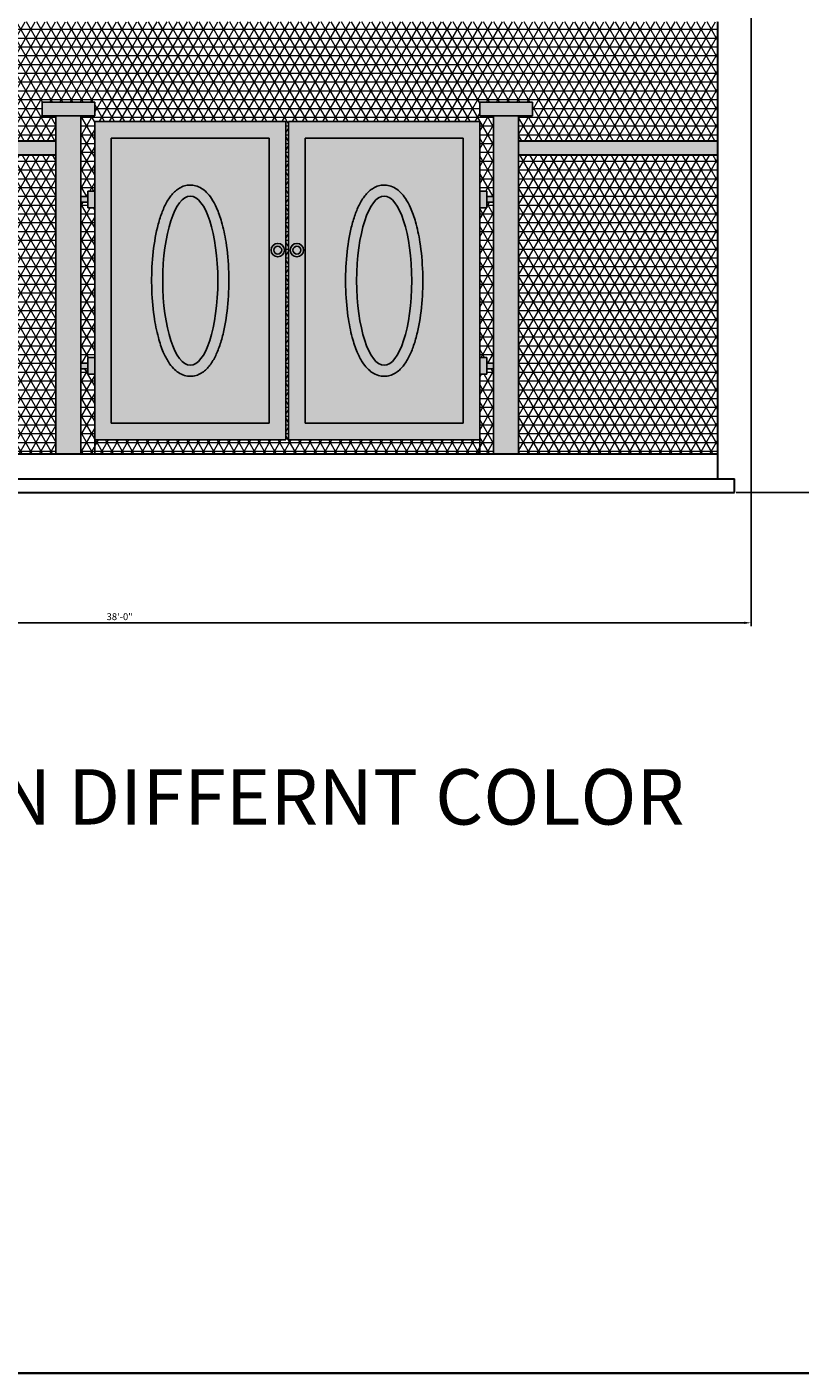
# Model space of a CAD drawing. Units: inches. Extents: x 2391 to 16591, y 7259 to 10239.
# Tile 4 of 27: x 3208 to 3487, y 7259 to 7745. Entities that reach past the tile are written whole.
import ezdxf

# ---------------------------------------------------------------- set-up
doc = ezdxf.new("R2010")
doc.units = ezdxf.units.IN
for name, color, linetype, lineweight in [('A-ANNO-DIMS', 4, 'Continuous', 18), ('A-ANNO-TITL', 3, 'Continuous', 30), ('A-ANNO-TTLB', 7, 'Continuous', 35), ('A-ELEV', 7, 'Continuous', 30), ('A-ELEV-GATE', 7, 'Continuous', 25), ('A-ELEV-GATE-PATT', 252, 'Continuous', 13), ('A-ELEV-PATT', 8, 'Continuous', 13), ('A-ELEV-SURF-PATT', 253, 'Continuous', 13)]:
    doc.layers.add(name, color=color, linetype=linetype, lineweight=lineweight)
doc.styles.get("Standard").update_dxf_attribs({"font": 'arial.ttf'})
doc.dimstyles.new('ISO-25', dxfattribs={"dimtxt": 2.5, "dimasz": 2.5, "dimexe": 1.25, "dimexo": 0.625, "dimtad": 1, "dimdec": 0, "dimlunit": 3, "dimtxsty": 'Standard', "dimcen": 2.5, "dimadec": 0, "dimazin": 0, "dimtfac": 1, "dimtdec": 0, "dimtmove": 0, "dimatfit": 3, "dimfxl": 1, "dimarcsym": 0})

# ---------------------------------------------------------------- blocks, each defined once
blk = doc.blocks.new('GATE-HINGE-ELEV')
for p, q in [((5, 6), (2.5, 6)), ((2.5, 6), (2.5, 0)), ((2.5, 4), (0, 4)), ((2.5, 2), (0, 2)), ((5, 0), (2.5, 0))]:
    blk.add_line(p, q)
blk = doc.blocks.new('*D83')
at = {"layer": 'A-ANNO-DIMS', "color": 0, "lineweight": -2, "transparency": 16777216}
for p, q in [((3013.78, 7751.89), (3013.78, 7528.22)), ((3469.78, 7751.89), (3469.78, 7528.22)), ((3016.28, 7529.47), (3467.28, 7529.47))]:
    blk.add_line(p, q, dxfattribs=at)
at = {"layer": 'A-ANNO-DIMS', "color": 0, "transparency": 16777216}
for points in [[(3016.28, 7529.89), (3016.28, 7529.05), (3013.78, 7529.47)], [(3467.28, 7529.89), (3467.28, 7529.05), (3469.78, 7529.47)]]:
    blk.add_solid(points, dxfattribs=at)
at = {"layer": 'Defpoints', "color": 0, "transparency": 16777216}
for p in [(3013.78, 7752.52), (3469.78, 7752.52), (3469.78, 7529.47)]:
    blk.add_point(p, dxfattribs=at)
at = {"layer": 'A-ANNO-DIMS', "color": 0, "transparency": 16777216, "insert": (3241.78, 7531.37), "char_height": 2.5, "attachment_point": 5}
blk.add_mtext('38\'-0"', dxfattribs=at)
blk = doc.blocks.new('*D84')
at = {"layer": 'A-ANNO-DIMS', "color": 0, "lineweight": -2, "transparency": 16777216}
for p, q in [((3437.4, 8339.52), (3518.08, 8339.52)), ((3516.83, 7579.02), (3516.83, 8337.02)), ((3464.4, 7576.52), (3518.08, 7576.52))]:
    blk.add_line(p, q, dxfattribs=at)
at = {"layer": 'A-ANNO-DIMS', "color": 0, "transparency": 16777216}
for points in [[(3516.41, 8337.02), (3517.24, 8337.02), (3516.83, 8339.52)], [(3516.41, 7579.02), (3517.24, 7579.02), (3516.83, 7576.52)]]:
    blk.add_solid(points, dxfattribs=at)
at = {"layer": 'Defpoints', "color": 0, "transparency": 16777216}
for p in [(3436.78, 8339.52), (3516.83, 8339.52), (3463.78, 7576.52)]:
    blk.add_point(p, dxfattribs=at)
at = {"layer": 'A-ANNO-DIMS', "color": 0, "transparency": 16777216, "insert": (3514.93, 7958.02), "char_height": 2.5, "attachment_point": 5, "rotation": 90}
blk.add_mtext('63\'-7"', dxfattribs=at)

msp = doc.modelspace()

# ---------------------------------------------------------------- hatches: boundary and pattern name
at = {"layer": 'A-ELEV-GATE-PATT'}
h = msp.add_hatch(color=256, dxfattribs=at)
h.dxf.hatch_style = 1
h.paths.add_polyline_path([(3218.78, 7590.52), (3227.78, 7590.52), (3227.78, 7712.52), (3218.78, 7712.52)])
h.paths.add_polyline_path([(3385.78, 7712.52), (3376.78, 7712.52), (3376.78, 7590.52), (3385.78, 7590.52)])
h = msp.add_hatch(color=256, dxfattribs=at)
h.dxf.hatch_style = 1
h.paths.add_polyline_path([(3232.78, 7595.52), (3301.78, 7595.52), (3301.78, 7710.52), (3232.78, 7710.52)])
h.paths.add_polyline_path([(3238.78, 7704.52), (3295.78, 7704.52), (3295.78, 7601.52), (3238.78, 7601.52)], flags=16)
edge = h.paths.add_edge_path(flags=0)
edge.add_spline(control_points=[(3267.28, 7618.48), (3267.98, 7618.48), (3268.69, 7618.59), (3270.01, 7618.97), (3270.63, 7619.25), (3271.76, 7619.93), (3272.28, 7620.32), (3273.23, 7621.18), (3273.67, 7621.64), (3274.89, 7623.14), (3275.59, 7624.27), (3276.85, 7626.76), (3277.41, 7628.13), (3278.43, 7631.09), (3278.88, 7632.69), (3280.01, 7637.55), (3280.54, 7641.06), (3281.19, 7648.39), (3281.29, 7652.22), (3281.06, 7659.76), (3280.73, 7663.47), (3279.77, 7669.53), (3279.25, 7671.99), (3278.08, 7676.08), (3277.48, 7677.78), (3276.25, 7680.54), (3275.65, 7681.66), (3274.42, 7683.5), (3273.83, 7684.25), (3272.61, 7685.46), (3272.01, 7685.95), (3270.68, 7686.77), (3269.94, 7687.11), (3268.5, 7687.48), (3267.83, 7687.57), (3266.48, 7687.55), (3265.81, 7687.44), (3264.54, 7687.06), (3263.95, 7686.8), (3262.86, 7686.16), (3262.36, 7685.79), (3261.44, 7684.98), (3261.02, 7684.54), (3259.81, 7683.1), (3259.11, 7682.01), (3257.84, 7679.59), (3257.28, 7678.26), (3256.26, 7675.38), (3255.81, 7673.83), (3254.67, 7669.1), (3254.11, 7665.68), (3253.42, 7658.51), (3253.28, 7654.75), (3253.43, 7647.32), (3253.72, 7643.64), (3254.6, 7637.46), (3255.12, 7634.88), (3256.27, 7630.6), (3256.87, 7628.82), (3258.1, 7625.93), (3258.7, 7624.75), (3259.92, 7622.82), (3260.52, 7622.04), (3261.74, 7620.77), (3262.33, 7620.25), (3263.67, 7619.38), (3264.41, 7619.01), (3265.88, 7618.59), (3266.58, 7618.48), (3267.28, 7618.48)], knot_values=[0, 0, 0, 0, 0.095196, 0.095196, 0.190392, 0.190392, 0.285588, 0.285588, 0.380784, 0.380784, 0.570897, 0.570897, 0.76101, 0.76101, 0.951123, 0.951123, 1.307609, 1.307609, 1.664096, 1.664096, 2.020583, 2.020583, 2.290036, 2.290036, 2.5108, 2.5108, 2.687191, 2.687191, 2.829292, 2.829292, 2.942747, 2.942747, 3.056202, 3.056202, 3.147245, 3.147245, 3.238288, 3.238288, 3.329331, 3.329331, 3.420374, 3.420374, 3.511418, 3.511418, 3.698581, 3.698581, 3.885745, 3.885745, 4.072908, 4.072908, 4.42383, 4.42383, 4.774752, 4.774752, 5.125674, 5.125674, 5.403289, 5.403289, 5.629501, 5.629501, 5.810378, 5.810378, 5.956164, 5.956164, 6.072402, 6.072402, 6.18864, 6.18864, 6.283185, 6.283185, 6.283185, 6.283185], degree=3, periodic=0)
edge = h.paths.add_edge_path(flags=0)
edge.add_ellipse((3267.28, 7653.02), major_axis=(0, -30.54), ratio=0.325581, start_angle=0, end_angle=360)
h.paths.add_polyline_path([(3300.28, 7664.05, -1), (3297.44, 7664.05, -1)], flags=16)
h.paths.add_polyline_path([(3302.78, 7595.52), (3371.78, 7595.52), (3371.78, 7710.52), (3302.78, 7710.52)])
h.paths.add_polyline_path([(3308.78, 7704.52), (3365.78, 7704.52), (3365.78, 7601.52), (3308.78, 7601.52)], flags=16)
edge = h.paths.add_edge_path(flags=0)
edge.add_spline(control_points=[(3337.28, 7618.48), (3337.98, 7618.48), (3338.69, 7618.59), (3340.01, 7618.97), (3340.63, 7619.25), (3341.76, 7619.93), (3342.28, 7620.32), (3343.23, 7621.18), (3343.67, 7621.64), (3344.89, 7623.14), (3345.59, 7624.27), (3346.85, 7626.76), (3347.41, 7628.13), (3348.43, 7631.09), (3348.88, 7632.69), (3350.01, 7637.55), (3350.54, 7641.06), (3351.19, 7648.39), (3351.29, 7652.22), (3351.06, 7659.76), (3350.73, 7663.47), (3349.77, 7669.53), (3349.25, 7671.99), (3348.08, 7676.08), (3347.48, 7677.78), (3346.25, 7680.54), (3345.65, 7681.66), (3344.42, 7683.5), (3343.83, 7684.25), (3342.61, 7685.46), (3342.01, 7685.95), (3340.68, 7686.77), (3339.94, 7687.11), (3338.5, 7687.48), (3337.83, 7687.57), (3336.48, 7687.55), (3335.81, 7687.44), (3334.54, 7687.06), (3333.95, 7686.8), (3332.86, 7686.16), (3332.36, 7685.79), (3331.44, 7684.98), (3331.02, 7684.54), (3329.81, 7683.1), (3329.11, 7682.01), (3327.84, 7679.59), (3327.28, 7678.26), (3326.26, 7675.38), (3325.81, 7673.83), (3324.67, 7669.1), (3324.11, 7665.68), (3323.42, 7658.51), (3323.28, 7654.75), (3323.43, 7647.32), (3323.72, 7643.64), (3324.6, 7637.46), (3325.12, 7634.88), (3326.27, 7630.6), (3326.87, 7628.82), (3328.1, 7625.93), (3328.7, 7624.75), (3329.92, 7622.82), (3330.52, 7622.04), (3331.74, 7620.77), (3332.33, 7620.25), (3333.67, 7619.38), (3334.41, 7619.01), (3335.88, 7618.59), (3336.58, 7618.48), (3337.28, 7618.48)], knot_values=[0, 0, 0, 0, 0.095196, 0.095196, 0.190392, 0.190392, 0.285588, 0.285588, 0.380784, 0.380784, 0.570897, 0.570897, 0.76101, 0.76101, 0.951123, 0.951123, 1.307609, 1.307609, 1.664096, 1.664096, 2.020583, 2.020583, 2.290036, 2.290036, 2.5108, 2.5108, 2.687191, 2.687191, 2.829292, 2.829292, 2.942747, 2.942747, 3.056202, 3.056202, 3.147245, 3.147245, 3.238288, 3.238288, 3.329331, 3.329331, 3.420374, 3.420374, 3.511418, 3.511418, 3.698581, 3.698581, 3.885745, 3.885745, 4.072908, 4.072908, 4.42383, 4.42383, 4.774752, 4.774752, 5.125674, 5.125674, 5.403289, 5.403289, 5.629501, 5.629501, 5.810378, 5.810378, 5.956164, 5.956164, 6.072402, 6.072402, 6.18864, 6.18864, 6.283185, 6.283185, 6.283185, 6.283185], degree=3, periodic=0)
edge = h.paths.add_edge_path(flags=0)
edge.add_ellipse((3337.28, 7653.02), major_axis=(0, -30.54), ratio=0.325581, start_angle=0, end_angle=360)
h.paths.add_polyline_path([(3308.19, 7664.05, -1), (3303.36, 7664.05, -1)], flags=16)
h.paths.add_polyline_path([(3307.19, 7664.05, -1), (3304.36, 7664.05, -1)], flags=0)
h = msp.add_hatch(color=256, dxfattribs=at)
h.dxf.hatch_style = 1
h.paths.add_polyline_path([(3238.78, 7704.52), (3238.78, 7601.52), (3295.78, 7601.52), (3295.78, 7704.52)])
edge = h.paths.add_edge_path(flags=16)
edge.add_spline(control_points=[(3267.28, 7618.48), (3267.98, 7618.48), (3268.69, 7618.59), (3270.01, 7618.97), (3270.63, 7619.25), (3271.76, 7619.93), (3272.28, 7620.32), (3273.23, 7621.18), (3273.67, 7621.64), (3274.89, 7623.14), (3275.59, 7624.27), (3276.85, 7626.76), (3277.41, 7628.13), (3278.43, 7631.09), (3278.88, 7632.69), (3280.01, 7637.55), (3280.54, 7641.06), (3281.19, 7648.39), (3281.29, 7652.22), (3281.06, 7659.76), (3280.73, 7663.47), (3279.77, 7669.53), (3279.25, 7671.99), (3278.08, 7676.08), (3277.48, 7677.78), (3276.25, 7680.54), (3275.65, 7681.66), (3274.42, 7683.5), (3273.83, 7684.25), (3272.61, 7685.46), (3272.01, 7685.95), (3270.68, 7686.77), (3269.94, 7687.11), (3268.5, 7687.48), (3267.83, 7687.57), (3266.48, 7687.55), (3265.81, 7687.44), (3264.54, 7687.06), (3263.95, 7686.8), (3262.86, 7686.16), (3262.36, 7685.79), (3261.44, 7684.98), (3261.02, 7684.54), (3259.81, 7683.1), (3259.11, 7682.01), (3257.84, 7679.59), (3257.28, 7678.26), (3256.26, 7675.38), (3255.81, 7673.83), (3254.67, 7669.1), (3254.11, 7665.68), (3253.42, 7658.51), (3253.28, 7654.75), (3253.43, 7647.32), (3253.72, 7643.64), (3254.6, 7637.46), (3255.12, 7634.88), (3256.27, 7630.6), (3256.87, 7628.82), (3258.1, 7625.93), (3258.7, 7624.75), (3259.92, 7622.82), (3260.52, 7622.04), (3261.74, 7620.77), (3262.33, 7620.25), (3263.67, 7619.38), (3264.41, 7619.01), (3265.88, 7618.59), (3266.58, 7618.48), (3267.28, 7618.48)], knot_values=[0, 0, 0, 0, 0.095196, 0.095196, 0.190392, 0.190392, 0.285588, 0.285588, 0.380784, 0.380784, 0.570897, 0.570897, 0.76101, 0.76101, 0.951123, 0.951123, 1.307609, 1.307609, 1.664096, 1.664096, 2.020583, 2.020583, 2.290036, 2.290036, 2.5108, 2.5108, 2.687191, 2.687191, 2.829292, 2.829292, 2.942747, 2.942747, 3.056202, 3.056202, 3.147245, 3.147245, 3.238288, 3.238288, 3.329331, 3.329331, 3.420374, 3.420374, 3.511418, 3.511418, 3.698581, 3.698581, 3.885745, 3.885745, 4.072908, 4.072908, 4.42383, 4.42383, 4.774752, 4.774752, 5.125674, 5.125674, 5.403289, 5.403289, 5.629501, 5.629501, 5.810378, 5.810378, 5.956164, 5.956164, 6.072402, 6.072402, 6.18864, 6.18864, 6.283185, 6.283185, 6.283185, 6.283185], degree=3, periodic=0)
edge = h.paths.add_edge_path(flags=0)
edge.add_ellipse((3267.28, 7653.02), major_axis=(0, -30.54), ratio=0.325581, start_angle=0, end_angle=360)
h.paths.add_polyline_path([(3308.78, 7704.52), (3308.78, 7601.52), (3365.78, 7601.52), (3365.78, 7704.52)])
edge = h.paths.add_edge_path(flags=16)
edge.add_spline(control_points=[(3337.28, 7618.48), (3337.98, 7618.48), (3338.69, 7618.59), (3340.01, 7618.97), (3340.63, 7619.25), (3341.76, 7619.93), (3342.28, 7620.32), (3343.23, 7621.18), (3343.67, 7621.64), (3344.89, 7623.14), (3345.59, 7624.27), (3346.85, 7626.76), (3347.41, 7628.13), (3348.43, 7631.09), (3348.88, 7632.69), (3350.01, 7637.55), (3350.54, 7641.06), (3351.19, 7648.39), (3351.29, 7652.22), (3351.06, 7659.76), (3350.73, 7663.47), (3349.77, 7669.53), (3349.25, 7671.99), (3348.08, 7676.08), (3347.48, 7677.78), (3346.25, 7680.54), (3345.65, 7681.66), (3344.42, 7683.5), (3343.83, 7684.25), (3342.61, 7685.46), (3342.01, 7685.95), (3340.68, 7686.77), (3339.94, 7687.11), (3338.5, 7687.48), (3337.83, 7687.57), (3336.48, 7687.55), (3335.81, 7687.44), (3334.54, 7687.06), (3333.95, 7686.8), (3332.86, 7686.16), (3332.36, 7685.79), (3331.44, 7684.98), (3331.02, 7684.54), (3329.81, 7683.1), (3329.11, 7682.01), (3327.84, 7679.59), (3327.28, 7678.26), (3326.26, 7675.38), (3325.81, 7673.83), (3324.67, 7669.1), (3324.11, 7665.68), (3323.42, 7658.51), (3323.28, 7654.75), (3323.43, 7647.32), (3323.72, 7643.64), (3324.6, 7637.46), (3325.12, 7634.88), (3326.27, 7630.6), (3326.87, 7628.82), (3328.1, 7625.93), (3328.7, 7624.75), (3329.92, 7622.82), (3330.52, 7622.04), (3331.74, 7620.77), (3332.33, 7620.25), (3333.67, 7619.38), (3334.41, 7619.01), (3335.88, 7618.59), (3336.58, 7618.48), (3337.28, 7618.48)], knot_values=[0, 0, 0, 0, 0.095196, 0.095196, 0.190392, 0.190392, 0.285588, 0.285588, 0.380784, 0.380784, 0.570897, 0.570897, 0.76101, 0.76101, 0.951123, 0.951123, 1.307609, 1.307609, 1.664096, 1.664096, 2.020583, 2.020583, 2.290036, 2.290036, 2.5108, 2.5108, 2.687191, 2.687191, 2.829292, 2.829292, 2.942747, 2.942747, 3.056202, 3.056202, 3.147245, 3.147245, 3.238288, 3.238288, 3.329331, 3.329331, 3.420374, 3.420374, 3.511418, 3.511418, 3.698581, 3.698581, 3.885745, 3.885745, 4.072908, 4.072908, 4.42383, 4.42383, 4.774752, 4.774752, 5.125674, 5.125674, 5.403289, 5.403289, 5.629501, 5.629501, 5.810378, 5.810378, 5.956164, 5.956164, 6.072402, 6.072402, 6.18864, 6.18864, 6.283185, 6.283185, 6.283185, 6.283185], degree=3, periodic=0)
edge = h.paths.add_edge_path(flags=0)
edge.add_ellipse((3337.28, 7653.02), major_axis=(0, -30.54), ratio=0.325581, start_angle=0, end_angle=360)
h = msp.add_hatch(color=256, dxfattribs=at)
h.dxf.hatch_style = 1
edge = h.paths.add_edge_path()
edge.add_spline(control_points=[(3267.28, 7618.48), (3267.98, 7618.48), (3268.69, 7618.59), (3270.01, 7618.97), (3270.63, 7619.25), (3271.76, 7619.93), (3272.28, 7620.32), (3273.23, 7621.18), (3273.67, 7621.64), (3274.89, 7623.14), (3275.59, 7624.27), (3276.85, 7626.76), (3277.41, 7628.13), (3278.43, 7631.09), (3278.88, 7632.69), (3280.01, 7637.55), (3280.54, 7641.06), (3281.19, 7648.39), (3281.29, 7652.22), (3281.06, 7659.76), (3280.73, 7663.47), (3279.77, 7669.53), (3279.25, 7671.99), (3278.08, 7676.08), (3277.48, 7677.78), (3276.25, 7680.54), (3275.65, 7681.66), (3274.42, 7683.5), (3273.83, 7684.25), (3272.61, 7685.46), (3272.01, 7685.95), (3270.68, 7686.77), (3269.94, 7687.11), (3268.5, 7687.48), (3267.83, 7687.57), (3266.48, 7687.55), (3265.81, 7687.44), (3264.54, 7687.06), (3263.95, 7686.8), (3262.86, 7686.16), (3262.36, 7685.79), (3261.44, 7684.98), (3261.02, 7684.54), (3259.81, 7683.1), (3259.11, 7682.01), (3257.84, 7679.59), (3257.28, 7678.26), (3256.26, 7675.38), (3255.81, 7673.83), (3254.67, 7669.1), (3254.11, 7665.68), (3253.42, 7658.51), (3253.28, 7654.75), (3253.43, 7647.32), (3253.72, 7643.64), (3254.6, 7637.46), (3255.12, 7634.88), (3256.27, 7630.6), (3256.87, 7628.82), (3258.1, 7625.93), (3258.7, 7624.75), (3259.92, 7622.82), (3260.52, 7622.04), (3261.74, 7620.77), (3262.33, 7620.25), (3263.67, 7619.38), (3264.41, 7619.01), (3265.88, 7618.59), (3266.58, 7618.48), (3267.28, 7618.48)], knot_values=[0, 0, 0, 0, 0.095196, 0.095196, 0.190392, 0.190392, 0.285588, 0.285588, 0.380784, 0.380784, 0.570897, 0.570897, 0.76101, 0.76101, 0.951123, 0.951123, 1.307609, 1.307609, 1.664096, 1.664096, 2.020583, 2.020583, 2.290036, 2.290036, 2.5108, 2.5108, 2.687191, 2.687191, 2.829292, 2.829292, 2.942747, 2.942747, 3.056202, 3.056202, 3.147245, 3.147245, 3.238288, 3.238288, 3.329331, 3.329331, 3.420374, 3.420374, 3.511418, 3.511418, 3.698581, 3.698581, 3.885745, 3.885745, 4.072908, 4.072908, 4.42383, 4.42383, 4.774752, 4.774752, 5.125674, 5.125674, 5.403289, 5.403289, 5.629501, 5.629501, 5.810378, 5.810378, 5.956164, 5.956164, 6.072402, 6.072402, 6.18864, 6.18864, 6.283185, 6.283185, 6.283185, 6.283185], degree=3, periodic=0)
edge = h.paths.add_edge_path(flags=16)
edge.add_ellipse((3267.28, 7653.02), major_axis=(0, -30.54), ratio=0.325581, start_angle=0, end_angle=360)
edge = h.paths.add_edge_path()
edge.add_spline(control_points=[(3337.28, 7618.48), (3337.98, 7618.48), (3338.69, 7618.59), (3340.01, 7618.97), (3340.63, 7619.25), (3341.76, 7619.93), (3342.28, 7620.32), (3343.23, 7621.18), (3343.67, 7621.64), (3344.89, 7623.14), (3345.59, 7624.27), (3346.85, 7626.76), (3347.41, 7628.13), (3348.43, 7631.09), (3348.88, 7632.69), (3350.01, 7637.55), (3350.54, 7641.06), (3351.19, 7648.39), (3351.29, 7652.22), (3351.06, 7659.76), (3350.73, 7663.47), (3349.77, 7669.53), (3349.25, 7671.99), (3348.08, 7676.08), (3347.48, 7677.78), (3346.25, 7680.54), (3345.65, 7681.66), (3344.42, 7683.5), (3343.83, 7684.25), (3342.61, 7685.46), (3342.01, 7685.95), (3340.68, 7686.77), (3339.94, 7687.11), (3338.5, 7687.48), (3337.83, 7687.57), (3336.48, 7687.55), (3335.81, 7687.44), (3334.54, 7687.06), (3333.95, 7686.8), (3332.86, 7686.16), (3332.36, 7685.79), (3331.44, 7684.98), (3331.02, 7684.54), (3329.81, 7683.1), (3329.11, 7682.01), (3327.84, 7679.59), (3327.28, 7678.26), (3326.26, 7675.38), (3325.81, 7673.83), (3324.67, 7669.1), (3324.11, 7665.68), (3323.42, 7658.51), (3323.28, 7654.75), (3323.43, 7647.32), (3323.72, 7643.64), (3324.6, 7637.46), (3325.12, 7634.88), (3326.27, 7630.6), (3326.87, 7628.82), (3328.1, 7625.93), (3328.7, 7624.75), (3329.92, 7622.82), (3330.52, 7622.04), (3331.74, 7620.77), (3332.33, 7620.25), (3333.67, 7619.38), (3334.41, 7619.01), (3335.88, 7618.59), (3336.58, 7618.48), (3337.28, 7618.48)], knot_values=[0, 0, 0, 0, 0.095196, 0.095196, 0.190392, 0.190392, 0.285588, 0.285588, 0.380784, 0.380784, 0.570897, 0.570897, 0.76101, 0.76101, 0.951123, 0.951123, 1.307609, 1.307609, 1.664096, 1.664096, 2.020583, 2.020583, 2.290036, 2.290036, 2.5108, 2.5108, 2.687191, 2.687191, 2.829292, 2.829292, 2.942747, 2.942747, 3.056202, 3.056202, 3.147245, 3.147245, 3.238288, 3.238288, 3.329331, 3.329331, 3.420374, 3.420374, 3.511418, 3.511418, 3.698581, 3.698581, 3.885745, 3.885745, 4.072908, 4.072908, 4.42383, 4.42383, 4.774752, 4.774752, 5.125674, 5.125674, 5.403289, 5.403289, 5.629501, 5.629501, 5.810378, 5.810378, 5.956164, 5.956164, 6.072402, 6.072402, 6.18864, 6.18864, 6.283185, 6.283185, 6.283185, 6.283185], degree=3, periodic=0)
edge = h.paths.add_edge_path(flags=16)
edge.add_ellipse((3337.28, 7653.02), major_axis=(0, -30.54), ratio=0.325581, start_angle=0, end_angle=360)
h = msp.add_hatch(color=256, dxfattribs=at)
h.dxf.hatch_style = 1
h.paths.add_polyline_path([(3232.78, 7685.36), (3230.28, 7685.36), (3230.28, 7679.36), (3232.78, 7679.36)])
h.paths.add_polyline_path([(3230.28, 7683.36), (3227.78, 7683.36), (3227.78, 7681.36), (3230.28, 7681.36)])
h.paths.add_polyline_path([(3230.28, 7623.23), (3227.78, 7623.23), (3227.78, 7621.23), (3230.28, 7621.23)])
h.paths.add_polyline_path([(3232.78, 7625.23), (3230.28, 7625.23), (3230.28, 7619.23), (3232.78, 7619.23)])
h.paths.add_polyline_path([(3376.78, 7683.36), (3374.28, 7683.36), (3374.28, 7681.36), (3376.78, 7681.36)])
h.paths.add_polyline_path([(3374.28, 7685.36), (3371.78, 7685.36), (3371.78, 7679.36), (3374.28, 7679.36)])
h.paths.add_polyline_path([(3374.28, 7625.23), (3371.78, 7625.23), (3371.78, 7619.23), (3374.28, 7619.23)])
h.paths.add_polyline_path([(3376.78, 7623.23), (3374.28, 7623.23), (3374.28, 7621.23), (3376.78, 7621.23)])
h = msp.add_hatch(color=256, dxfattribs=at)
h.dxf.hatch_style = 1
edge = h.paths.add_edge_path()
edge.add_ellipse((3267.28, 7653.02), major_axis=(0, -30.54), ratio=0.325581, start_angle=0, end_angle=360)
edge = h.paths.add_edge_path()
edge.add_ellipse((3337.28, 7653.02), major_axis=(0, -30.54), ratio=0.325581, start_angle=0, end_angle=360)
h = msp.add_hatch(color=256, dxfattribs=at)
h.dxf.hatch_style = 1
h.paths.add_polyline_path([(3301.28, 7664.05, 1), (3296.44, 7664.05, 1)])
h.paths.add_polyline_path([(3300.28, 7664.05, 1), (3297.44, 7664.05, 1)], flags=16)
h.paths.add_polyline_path([(3308.19, 7664.05, 1), (3303.36, 7664.05, 1)])
h.paths.add_polyline_path([(3307.19, 7664.05, 1), (3304.36, 7664.05, 1)], flags=16)
h = msp.add_hatch(color=256, dxfattribs=at)
h.dxf.hatch_style = 1
h.paths.add_polyline_path([(3300.28, 7664.05, 1), (3297.44, 7664.05, 1)])
h.paths.add_polyline_path([(3307.19, 7664.05, 1), (3304.36, 7664.05, 1)])
at = {"layer": 'A-ELEV-PATT'}
h = msp.add_hatch(dxfattribs=at)
h.set_pattern_fill('NET3', color=256)
h.paths.add_polyline_path([(3457.78, 8232.52), (3339.28, 8232.52), (3339.28, 8076.52), (3457.78, 8076.52)])
h.paths.add_polyline_path([(3415.03, 8124.52), (3373.03, 8124.52), (3373.03, 8178.52), (3415.03, 8178.52)], flags=16)
h.paths.add_polyline_path([(3412.03, 8127.52), (3376.03, 8127.52), (3376.03, 8175.52), (3412.03, 8175.52)], flags=0)
h.paths.add_polyline_path([(3457.78, 8070.52), (3339.28, 8070.52), (3339.28, 7914.52), (3457.78, 7914.52)])
h.paths.add_polyline_path([(3415.03, 7962.52), (3373.03, 7962.52), (3373.03, 8016.52), (3415.03, 8016.52)], flags=16)
h.paths.add_polyline_path([(3412.03, 7965.52), (3376.03, 7965.52), (3376.03, 8013.52), (3412.03, 8013.52)], flags=0)
h.paths.add_polyline_path([(3457.78, 7908.52), (3339.28, 7908.52), (3339.28, 7752.52), (3457.78, 7752.52)])
h.paths.add_polyline_path([(3415.03, 7800.52), (3373.03, 7800.52), (3373.03, 7854.52), (3415.03, 7854.52)], flags=16)
h.paths.add_polyline_path([(3412.03, 7803.52), (3376.03, 7803.52), (3376.03, 7851.52), (3412.03, 7851.52)], flags=0)
h.paths.add_polyline_path([(3339.28, 8232.52), (3227.28, 8232.52), (3227.28, 8076.52), (3339.28, 8076.52)])
h.paths.add_polyline_path([(3260.28, 8124.52), (3260.28, 8178.52), (3302.28, 8178.52), (3302.28, 8124.52)], flags=16)
h.paths.add_polyline_path([(3263.28, 8127.52), (3263.28, 8175.52), (3299.28, 8175.52), (3299.28, 8127.52)], flags=0)
h.paths.add_polyline_path([(3339.28, 8070.52), (3227.28, 8070.52), (3227.28, 7914.52), (3339.28, 7914.52)])
h.paths.add_polyline_path([(3260.28, 8016.52), (3302.28, 8016.52), (3302.28, 7962.52), (3260.28, 7962.52)], flags=16)
h.paths.add_polyline_path([(3263.28, 8013.52), (3299.28, 8013.52), (3299.28, 7965.52), (3263.28, 7965.52)], flags=0)
h.paths.add_polyline_path([(3339.28, 7908.52), (3227.28, 7908.52), (3227.28, 7752.52), (3339.28, 7752.52)])
h.paths.add_polyline_path([(3260.28, 7854.52), (3302.28, 7854.52), (3302.28, 7800.52), (3260.28, 7800.52)], flags=16)
h.paths.add_polyline_path([(3263.28, 7851.52), (3299.28, 7851.52), (3299.28, 7803.52), (3263.28, 7803.52)], flags=0)
h.paths.add_polyline_path([(3213.78, 7717.52), (3232.78, 7717.52), (3232.78, 7712.52), (3227.78, 7712.52), (3227.78, 7683.36), (3230.28, 7683.36), (3230.28, 7685.36), (3232.78, 7685.36), (3232.78, 7710.52), (3301.78, 7710.52), (3301.78, 7595.52), (3232.78, 7595.52), (3232.78, 7590.52), (3371.78, 7590.52), (3371.78, 7595.52), (3302.78, 7595.52), (3302.78, 7710.52), (3371.78, 7710.52), (3371.78, 7685.36), (3374.28, 7685.36), (3374.28, 7683.36), (3376.78, 7683.36), (3376.78, 7712.52), (3371.78, 7712.52), (3371.78, 7717.52), (3390.78, 7717.52), (3390.78, 7712.52), (3385.78, 7712.52), (3385.78, 7703.52), (3457.78, 7703.52), (3457.78, 7746.52), (3025.78, 7746.52), (3025.78, 7703.52), (3218.78, 7703.52), (3218.78, 7712.52), (3213.78, 7712.52)])
h.paths.add_polyline_path([(3232.78, 7679.36), (3230.28, 7679.36), (3230.28, 7681.36), (3227.78, 7681.36), (3227.78, 7623.23), (3230.28, 7623.23), (3230.28, 7625.23), (3232.78, 7625.23)], flags=17)
h.paths.add_polyline_path([(3232.78, 7619.23), (3230.28, 7619.23), (3230.28, 7621.23), (3227.78, 7621.23), (3227.78, 7590.52), (3232.78, 7590.52)], flags=17)
h.paths.add_polyline_path([(3376.78, 7681.36), (3374.28, 7681.36), (3374.28, 7679.36), (3371.78, 7679.36), (3371.78, 7625.23), (3374.28, 7625.23), (3374.28, 7623.23), (3376.78, 7623.23)], flags=17)
h.paths.add_polyline_path([(3376.78, 7621.23), (3374.28, 7621.23), (3374.28, 7619.23), (3371.78, 7619.23), (3371.78, 7590.52), (3376.78, 7590.52)], flags=17)
h = msp.add_hatch(dxfattribs=at)
h.set_pattern_fill('NET3', color=256)
h.paths.add_polyline_path([(3218.78, 7590.52), (3218.78, 7698.52), (3025.78, 7698.52), (3025.78, 7590.52)])
h.paths.add_polyline_path([(3457.78, 7698.52), (3385.78, 7698.52), (3385.78, 7590.52), (3457.78, 7590.52)])
at = {"layer": 'A-ELEV-SURF-PATT'}
h = msp.add_hatch(color=256, dxfattribs=at)
h.dxf.hatch_style = 1
h.paths.add_polyline_path([(3218.78, 7698.52), (3218.78, 7703.52), (3025.78, 7703.52), (3025.78, 7698.52)])
h.paths.add_polyline_path([(3213.78, 7717.52), (3213.78, 7712.52), (3232.78, 7712.52), (3232.78, 7717.52)])
h.paths.add_polyline_path([(3371.78, 7717.52), (3371.78, 7712.52), (3390.78, 7712.52), (3390.78, 7717.52)])
h.paths.add_polyline_path([(3385.78, 7703.52), (3385.78, 7698.52), (3457.78, 7698.52), (3457.78, 7703.52)])

# ---------------------------------------------------------------- linework, layer by layer
at = {"layer": 'A-ANNO-TTLB'}
msp.add_lwpolyline([(2391.28, 10239.38), (4154.2, 10239.38), (4154.2, 7258.54), (2391.28, 7258.54)], close=True, dxfattribs=at)
at = {"layer": 'A-ELEV'}
for p, q in [((3457.78, 7581.52), (3457.78, 7746.52)), ((3025.78, 7703.52), (3218.78, 7703.52)), ((3385.78, 7703.52), (3457.78, 7703.52)), ((3025.78, 7698.52), (3218.78, 7698.52)), ((3385.78, 7698.52), (3457.78, 7698.52)), ((3025.78, 7590.52), (3457.78, 7590.52)), ((3019.78, 7581.52), (3463.78, 7581.52)), ((3463.78, 7576.52), (3463.78, 7581.52)), ((3019.78, 7576.52), (3463.78, 7576.52))]:
    msp.add_line(p, q, dxfattribs=at)
at = {"layer": 'A-ELEV-GATE'}
for p, q in [((3213.78, 7712.52), (3213.78, 7717.52)), ((3232.78, 7717.52), (3213.78, 7717.52)), ((3232.78, 7712.52), (3232.78, 7717.52)), ((3371.78, 7712.52), (3371.78, 7717.52)), ((3371.78, 7717.52), (3390.78, 7717.52)), ((3390.78, 7712.52), (3390.78, 7717.52)), ((3232.78, 7712.52), (3213.78, 7712.52)), ((3218.78, 7590.52), (3218.78, 7712.52)), ((3227.78, 7590.52), (3227.78, 7712.52)), ((3232.78, 7590.52), (3232.78, 7710.52)), ((3232.78, 7710.52), (3301.78, 7710.52)), ((3301.78, 7710.52), (3301.78, 7595.52)), ((3302.78, 7710.52), (3371.78, 7710.52)), ((3302.78, 7710.52), (3302.78, 7595.52)), ((3371.78, 7712.52), (3390.78, 7712.52)), ((3371.78, 7590.52), (3371.78, 7710.52)), ((3376.78, 7590.52), (3376.78, 7712.52)), ((3385.78, 7590.52), (3385.78, 7712.52)), ((3238.78, 7601.52), (3238.78, 7704.52)), ((3238.78, 7704.52), (3295.78, 7704.52)), ((3295.78, 7704.52), (3295.78, 7601.52)), ((3308.78, 7704.52), (3365.78, 7704.52)), ((3308.78, 7704.52), (3308.78, 7601.52)), ((3365.78, 7601.52), (3365.78, 7704.52)), ((3238.78, 7601.52), (3295.78, 7601.52)), ((3308.78, 7601.52), (3365.78, 7601.52)), ((3232.78, 7595.52), (3301.78, 7595.52)), ((3302.78, 7595.52), (3371.78, 7595.52))]:
    msp.add_line(p, q, dxfattribs=at)
for centre, radius in [((3298.86, 7664.05), 2.42), ((3305.77, 7664.05), 2.42), ((3298.86, 7664.05), 1.42), ((3305.77, 7664.05), 1.42)]:
    msp.add_circle(centre, radius, dxfattribs=at)
for centre in [(3267.28, 7653.02), (3337.28, 7653.02)]:
    msp.add_ellipse(centre, major_axis=(0, -30.54), ratio=0.325581, dxfattribs=at)
for points in [[(3267.28, 7618.48), (3267.98, 7618.48), (3268.69, 7618.59), (3270.01, 7618.97), (3270.63, 7619.25), (3271.76, 7619.93), (3272.28, 7620.32), (3273.23, 7621.18), (3273.67, 7621.64), (3274.89, 7623.14), (3275.59, 7624.27), (3276.85, 7626.76), (3277.41, 7628.13), (3278.43, 7631.09), (3278.88, 7632.69), (3280.01, 7637.55), (3280.54, 7641.06), (3281.19, 7648.39), (3281.29, 7652.22), (3281.06, 7659.76), (3280.73, 7663.47), (3279.77, 7669.53), (3279.25, 7671.99), (3278.08, 7676.08), (3277.48, 7677.78), (3276.25, 7680.54), (3275.65, 7681.66), (3274.42, 7683.5), (3273.83, 7684.25), (3272.61, 7685.46), (3272.01, 7685.95), (3270.68, 7686.77), (3269.94, 7687.11), (3268.5, 7687.48), (3267.83, 7687.57), (3266.48, 7687.55), (3265.81, 7687.44), (3264.54, 7687.06), (3263.95, 7686.8), (3262.86, 7686.16), (3262.36, 7685.79), (3261.44, 7684.98), (3261.02, 7684.54), (3259.81, 7683.1), (3259.11, 7682.01), (3257.84, 7679.59), (3257.28, 7678.26), (3256.26, 7675.38), (3255.81, 7673.83), (3254.67, 7669.1), (3254.11, 7665.68), (3253.42, 7658.51), (3253.28, 7654.75), (3253.43, 7647.32), (3253.72, 7643.64), (3254.6, 7637.46), (3255.12, 7634.88), (3256.27, 7630.6), (3256.87, 7628.82), (3258.1, 7625.93), (3258.7, 7624.75), (3259.92, 7622.82), (3260.52, 7622.04), (3261.74, 7620.77), (3262.33, 7620.25), (3263.67, 7619.38), (3264.41, 7619.01), (3265.88, 7618.59), (3266.58, 7618.48), (3267.28, 7618.48)], [(3337.28, 7618.48), (3337.98, 7618.48), (3338.69, 7618.59), (3340.01, 7618.97), (3340.63, 7619.25), (3341.76, 7619.93), (3342.28, 7620.32), (3343.23, 7621.18), (3343.67, 7621.64), (3344.89, 7623.14), (3345.59, 7624.27), (3346.85, 7626.76), (3347.41, 7628.13), (3348.43, 7631.09), (3348.88, 7632.69), (3350.01, 7637.55), (3350.54, 7641.06), (3351.19, 7648.39), (3351.29, 7652.22), (3351.06, 7659.76), (3350.73, 7663.47), (3349.77, 7669.53), (3349.25, 7671.99), (3348.08, 7676.08), (3347.48, 7677.78), (3346.25, 7680.54), (3345.65, 7681.66), (3344.42, 7683.5), (3343.83, 7684.25), (3342.61, 7685.46), (3342.01, 7685.95), (3340.68, 7686.77), (3339.94, 7687.11), (3338.5, 7687.48), (3337.83, 7687.57), (3336.48, 7687.55), (3335.81, 7687.44), (3334.54, 7687.06), (3333.95, 7686.8), (3332.86, 7686.16), (3332.36, 7685.79), (3331.44, 7684.98), (3331.02, 7684.54), (3329.81, 7683.1), (3329.11, 7682.01), (3327.84, 7679.59), (3327.28, 7678.26), (3326.26, 7675.38), (3325.81, 7673.83), (3324.67, 7669.1), (3324.11, 7665.68), (3323.42, 7658.51), (3323.28, 7654.75), (3323.43, 7647.32), (3323.72, 7643.64), (3324.6, 7637.46), (3325.12, 7634.88), (3326.27, 7630.6), (3326.87, 7628.82), (3328.1, 7625.93), (3328.7, 7624.75), (3329.92, 7622.82), (3330.52, 7622.04), (3331.74, 7620.77), (3332.33, 7620.25), (3333.67, 7619.38), (3334.41, 7619.01), (3335.88, 7618.59), (3336.58, 7618.48), (3337.28, 7618.48)]]:
    msp.add_open_spline(points, degree=3, knots=[0, 0, 0, 0, 0.095196, 0.095196, 0.190392, 0.190392, 0.285588, 0.285588, 0.380784, 0.380784, 0.570897, 0.570897, 0.76101, 0.76101, 0.951123, 0.951123, 1.307609, 1.307609, 1.664096, 1.664096, 2.020583, 2.020583, 2.290036, 2.290036, 2.5108, 2.5108, 2.687191, 2.687191, 2.829292, 2.829292, 2.942747, 2.942747, 3.056202, 3.056202, 3.147245, 3.147245, 3.238288, 3.238288, 3.329331, 3.329331, 3.420374, 3.420374, 3.511418, 3.511418, 3.698581, 3.698581, 3.885745, 3.885745, 4.072908, 4.072908, 4.42383, 4.42383, 4.774752, 4.774752, 5.125674, 5.125674, 5.403289, 5.403289, 5.629501, 5.629501, 5.810378, 5.810378, 5.956164, 5.956164, 6.072402, 6.072402, 6.18864, 6.18864, 6.283185, 6.283185, 6.283185, 6.283185], dxfattribs=at)

# ---------------------------------------------------------------- block references
for p in [(3227.78, 7679.36), (3227.78, 7619.23)]:
    msp.add_blockref('GATE-HINGE-ELEV', p, dxfattribs=at)
at = {"layer": 'A-ELEV-GATE', "rotation": 180}
for p in [(3376.78, 7685.36), (3376.78, 7625.23)]:
    msp.add_blockref('GATE-HINGE-ELEV', p, dxfattribs=at)

# ---------------------------------------------------------------- texts
at = {"layer": 'A-ANNO-TITL', "insert": (2944.88, 7476.61), "char_height": 20, "attachment_point": 1}
msp.add_mtext_dynamic_manual_height_columns('FRONT ELEVATION IN DIFFERNT COLOR', width=1534.7599, gutter_width=12.5, heights=[0], dxfattribs=at)

# ---------------------------------------------------------------- dimensions: what is measured, and where the dimension line sits
at = {"layer": 'A-ANNO-DIMS'}
dim = msp.add_linear_dim(base=(3516.83, 8339.52), p1=(3463.78, 7576.52), p2=(3436.78, 8339.52), angle=90, dimstyle='ISO-25', override={"dimdec": 1, "dimlfac": 1, "dimrnd": 0, "dimzin": 1, "dimdsep": 46, "dimlunit": 4, "dimfrac": 2}, dxfattribs=at)
dim.commit()
dim.dimension.update_dxf_attribs({"geometry": '*D84', "text_midpoint": (3514.93, 7958.02)})
dim = msp.add_linear_dim(base=(3469.78, 7529.47), p1=(3013.78, 7752.52), p2=(3469.78, 7752.52), dimstyle='ISO-25', override={"dimdec": 1, "dimlfac": 1, "dimrnd": 0, "dimzin": 1, "dimdsep": 46, "dimlunit": 4, "dimfrac": 2}, dxfattribs=at)
dim.commit()
dim.dimension.update_dxf_attribs({"geometry": '*D83', "text_midpoint": (3241.78, 7531.37)})

doc.saveas('drawing.dxf')
